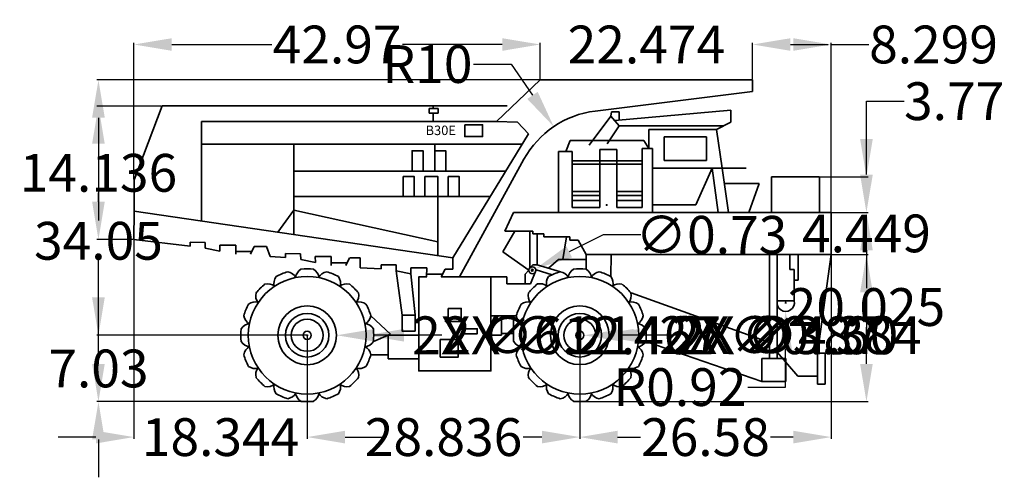
# Model space of a CAD drawing. Units: millimetres. Extents: x 52 to 156, y 12 to 60.
import ezdxf

# ---------------------------------------------------------------- set-up
doc = ezdxf.new("R2010")
doc.units = ezdxf.units.MM
doc.header["$MEASUREMENT"] = 0
for name, color, linetype, lineweight in [('M-DIMS', 2, 'Continuous', 18), ('M-OUTL', 7, 'Continuous', 35), ('M-TEXT', 3, 'Continuous', 25), ('M-WHEL', 8, 'Continuous', 35)]:
    doc.layers.add(name, color=color, linetype=linetype, lineweight=lineweight)
doc.styles.get("Standard").update_dxf_attribs({"font": 'arial.ttf'})
doc.dimstyles.get("Standard").update_dxf_attribs({"dimtxt": 4, "dimasz": 4, "dimexe": 0.18, "dimexo": 0.0625, "dimgap": 0.09, "dimtad": 0, "dimtih": 1, "dimtoh": 1, "dimdec": 0, "dimzin": 0, "dimdsep": 46, "dimtxsty": 'Standard', "dimcen": 0.09, "dimadec": 0, "dimazin": 0, "dimtfac": 1, "dimtdec": 0, "dimtofl": 0, "dimtmove": 0, "dimatfit": 3, "dimfxl": 1, "dimtolj": 1, "dimtzin": 0, "dimarcsym": 0})

# ---------------------------------------------------------------- blocks, each defined once
blk = doc.blocks.new('*U3')
for p, q in [((-6.73, -0.78), (-6.43, 0.09)), ((-4.89, 0.27), (-4.78, -0.69)), ((-3.11, -0.49), (-3.19, 0.15)), ((-3.19, 0.15), (-1.61, 0.02)), ((-1.61, 0.02), (-1.53, -0.6)), ((0.05, -0.42), (0, 0)), ((-4.86, -0.01), (-6.54, -0.21)), ((-4.78, -0.69), (-3.11, -0.49)), ((-1.53, -0.6), (0.05, -0.42))]:
    blk.add_line(p, q)
blk = doc.blocks.new('*U4')
at = {"layer": 'M-OUTL', "color": 0, "linetype": 'ByBlock', "lineweight": -2, "transparency": 16777216, "rotation": 173.2489355326982}
for p in [(70.14, 36.17), (80.23, 34.97), (90.33, 33.78)]:
    blk.add_blockref('*U3', p, dxfattribs=at)
blk = doc.blocks.new('*U1')
for centre, radius, start, end in [((0, -0.63), 1.25, 122.4091, 172.2725), ((0, -6.57), 7.03, 84.5202, 95.4798), ((0, -0.63), 1.25, 7.7275, 57.5909)]:
    blk.add_arc(centre, radius, start, end)
blk = doc.blocks.new('*U2')
at = {"color": 0, "linetype": 'ByBlock', "lineweight": -2, "transparency": 16777216}
for p, rotation in [((21.9, 20.49), 22.49999999999999), ((26.93, 20.49), 337.5), ((19.77, 19.07), 45.00000000000001), ((29.06, 19.07), 315), ((18.35, 16.94), 67.5), ((30.49, 16.94), 292.5), ((17.85, 14.43), 90), ((30.99, 14.43), 270), ((18.35, 11.91), 112.5), ((30.49, 11.91), 247.5), ((19.77, 9.78), 135), ((29.06, 9.78), 225), ((21.9, 8.36), 157.5), ((26.93, 8.36), 202.4999999999999), ((24.42, 7.86), 180)]:
    blk.add_blockref('*U1', p, dxfattribs=dict(at, rotation=rotation))
blk.add_blockref('*U1', (24.42, 21), dxfattribs=at)
blk = doc.blocks.new('WHEEL-TYRE')
for radius in [6.23, 3.11, 2.3, 1.69, 0.434]:
    blk.add_circle((6.23, 6.23), radius)
blk.add_blockref('*U2', (-18.18, -8.19))
blk = doc.blocks.new('*D6')
at = {"layer": 'Defpoints', "color": 0, "transparency": 16777216}
for p in [(107.16, 57.52), (107.16, 53.77), (64.19, 43.2)]:
    blk.add_point(p, dxfattribs=at)
at = {"layer": 'M-DIMS', "color": 0, "lineweight": -2, "transparency": 16777216}
for p, q in [((64.19, 43.26), (64.19, 57.7)), ((68.19, 57.52), (78.76, 57.52)), ((103.16, 57.52), (92.6, 57.52)), ((107.16, 53.84), (107.16, 57.7))]:
    blk.add_line(p, q, dxfattribs=at)
at = {"layer": 'M-DIMS', "color": 0, "transparency": 16777216}
for points in [[(68.19, 58.18), (68.19, 56.85), (64.19, 57.52)], [(103.16, 58.18), (103.16, 56.85), (107.16, 57.52)]]:
    blk.add_solid(points, dxfattribs=at)
at = {"layer": 'M-DIMS', "color": 0, "transparency": 16777216, "insert": (85.68, 57.52), "char_height": 4, "attachment_point": 5}
blk.add_mtext('\\A1;42.97', dxfattribs=at)
blk = doc.blocks.new('*D7')
at = {"layer": 'Defpoints', "color": 0, "transparency": 16777216}
for p in [(129.64, 57.52), (107.16, 53.77), (129.64, 53.77)]:
    blk.add_point(p, dxfattribs=at)
at = {"layer": 'M-DIMS', "color": 0, "lineweight": -2, "transparency": 16777216}
for p, q in [((103.16, 57.52), (99.16, 57.52)), ((107.16, 53.84), (107.16, 57.7)), ((129.64, 53.84), (129.64, 57.7)), ((133.64, 57.52), (137.64, 57.52))]:
    blk.add_line(p, q, dxfattribs=at)
at = {"layer": 'M-DIMS', "color": 0, "transparency": 16777216}
for points in [[(103.16, 58.18), (103.16, 56.85), (107.16, 57.52)], [(133.64, 58.18), (133.64, 56.85), (129.64, 57.52)]]:
    blk.add_solid(points, dxfattribs=at)
at = {"layer": 'M-DIMS', "color": 0, "transparency": 16777216, "insert": (118.4, 57.52), "char_height": 4, "attachment_point": 5}
blk.add_mtext('\\A1;22.474', dxfattribs=at)
blk = doc.blocks.new('*D8')
at = {"layer": 'Defpoints', "color": 0, "transparency": 16777216}
for p in [(137.94, 57.52), (129.64, 53.77), (137.94, 39.75)]:
    blk.add_point(p, dxfattribs=at)
at = {"layer": 'M-DIMS', "color": 0, "lineweight": -2, "transparency": 16777216}
for p, q in [((129.64, 53.84), (129.64, 57.7)), ((133.64, 57.52), (133.94, 57.52)), ((137.94, 39.81), (137.94, 57.7)), ((137.94, 57.52), (141.94, 57.52))]:
    blk.add_line(p, q, dxfattribs=at)
at = {"layer": 'M-DIMS', "color": 0, "transparency": 16777216}
for points in [[(133.64, 58.18), (133.64, 56.85), (129.64, 57.52)], [(133.94, 58.18), (133.94, 56.85), (137.94, 57.52)]]:
    blk.add_solid(points, dxfattribs=at)
at = {"layer": 'M-DIMS', "color": 0, "transparency": 16777216, "insert": (148.78, 57.52), "char_height": 4, "attachment_point": 5}
blk.add_mtext('\\A1;8.299', dxfattribs=at)
blk = doc.blocks.new('*D9')
at = {"layer": 'Defpoints', "color": 0, "transparency": 16777216}
for p in [(64.17, 36.88), (82.52, 26.75), (82.52, 15.98)]:
    blk.add_point(p, dxfattribs=at)
at = {"layer": 'M-DIMS', "color": 0, "lineweight": -2, "transparency": 16777216}
for p, q in [((64.17, 36.81), (64.17, 15.8)), ((82.52, 26.69), (82.52, 15.8)), ((60.17, 15.98), (56.17, 15.98)), ((86.52, 15.98), (90.52, 15.98))]:
    blk.add_line(p, q, dxfattribs=at)
at = {"layer": 'M-DIMS', "color": 0, "transparency": 16777216}
for points in [[(60.17, 16.65), (60.17, 15.31), (64.17, 15.98)], [(86.52, 16.65), (86.52, 15.31), (82.52, 15.98)]]:
    blk.add_solid(points, dxfattribs=at)
at = {"layer": 'M-DIMS', "color": 0, "transparency": 16777216, "insert": (73.35, 15.98), "char_height": 4, "attachment_point": 5}
blk.add_mtext('\\A1;18.344', dxfattribs=at)
blk = doc.blocks.new('*D10')
at = {"layer": 'Defpoints', "color": 0, "transparency": 16777216}
for p in [(82.52, 26.75), (111.35, 26.75), (111.35, 15.98)]:
    blk.add_point(p, dxfattribs=at)
at = {"layer": 'M-DIMS', "color": 0, "lineweight": -2, "transparency": 16777216}
for p, q in [((82.52, 26.69), (82.52, 15.8)), ((111.35, 26.69), (111.35, 15.8)), ((86.52, 15.98), (88.51, 15.98)), ((107.35, 15.98), (105.36, 15.98))]:
    blk.add_line(p, q, dxfattribs=at)
at = {"layer": 'M-DIMS', "color": 0, "transparency": 16777216}
for points in [[(86.52, 16.65), (86.52, 15.31), (82.52, 15.98)], [(107.35, 16.65), (107.35, 15.31), (111.35, 15.98)]]:
    blk.add_solid(points, dxfattribs=at)
at = {"layer": 'M-DIMS', "color": 0, "transparency": 16777216, "insert": (96.94, 15.98), "char_height": 4, "attachment_point": 5}
blk.add_mtext('\\A1;28.836', dxfattribs=at)
blk = doc.blocks.new('*D11')
at = {"layer": 'Defpoints', "color": 0, "transparency": 16777216}
for p in [(137.94, 35.3), (111.35, 26.75), (137.94, 15.98)]:
    blk.add_point(p, dxfattribs=at)
at = {"layer": 'M-DIMS', "color": 0, "lineweight": -2, "transparency": 16777216}
for p, q in [((137.94, 35.24), (137.94, 15.8)), ((111.35, 26.69), (111.35, 15.8)), ((115.35, 15.98), (117.77, 15.98)), ((133.94, 15.98), (131.52, 15.98))]:
    blk.add_line(p, q, dxfattribs=at)
at = {"layer": 'M-DIMS', "color": 0, "transparency": 16777216}
for points in [[(115.35, 16.65), (115.35, 15.31), (111.35, 15.98)], [(133.94, 16.65), (133.94, 15.31), (137.94, 15.98)]]:
    blk.add_solid(points, dxfattribs=at)
at = {"layer": 'M-DIMS', "color": 0, "transparency": 16777216, "insert": (124.65, 15.98), "char_height": 4, "attachment_point": 5}
blk.add_mtext('\\A1;26.58', dxfattribs=at)
blk = doc.blocks.new('*D12')
at = {"layer": 'Defpoints', "color": 0, "transparency": 16777216}
for p in [(60.43, 53.77), (107.16, 53.77), (82.52, 19.73)]:
    blk.add_point(p, dxfattribs=at)
at = {"layer": 'M-DIMS', "color": 0, "lineweight": -2, "transparency": 16777216}
for p, q in [((107.1, 53.77), (60.25, 53.77)), ((60.43, 49.77), (60.43, 38.88)), ((60.43, 23.73), (60.43, 34.62)), ((82.46, 19.73), (60.25, 19.73))]:
    blk.add_line(p, q, dxfattribs=at)
at = {"layer": 'M-DIMS', "color": 0, "transparency": 16777216}
for points in [[(59.76, 49.77), (61.1, 49.77), (60.43, 53.77)], [(59.76, 23.73), (61.1, 23.73), (60.43, 19.73)]]:
    blk.add_solid(points, dxfattribs=at)
at = {"layer": 'M-DIMS', "color": 0, "transparency": 16777216, "insert": (60.43, 36.75), "char_height": 4, "attachment_point": 5}
blk.add_mtext('\\A1;34.05', dxfattribs=at)
blk = doc.blocks.new('*D13')
at = {"layer": 'Defpoints', "color": 0, "transparency": 16777216}
for p in [(60.43, 26.75), (82.52, 26.75), (82.52, 19.73)]:
    blk.add_point(p, dxfattribs=at)
at = {"layer": 'M-DIMS', "color": 0, "lineweight": -2, "transparency": 16777216}
for p, q in [((60.43, 30.75), (60.43, 34.75)), ((82.46, 26.75), (60.25, 26.75)), ((82.46, 19.73), (60.25, 19.73)), ((60.43, 15.73), (60.43, 11.73))]:
    blk.add_line(p, q, dxfattribs=at)
at = {"layer": 'M-DIMS', "color": 0, "transparency": 16777216}
for points in [[(59.76, 30.75), (61.1, 30.75), (60.43, 26.75)], [(59.76, 15.73), (61.1, 15.73), (60.43, 19.73)]]:
    blk.add_solid(points, dxfattribs=at)
at = {"layer": 'M-DIMS', "color": 0, "transparency": 16777216, "insert": (60.43, 23.24), "char_height": 4, "attachment_point": 5}
blk.add_mtext('\\A1;7.03', dxfattribs=at)
blk = doc.blocks.new('*D14')
at = {"layer": 'Defpoints', "color": 0, "transparency": 16777216}
for p in [(60.43, 51.01), (67.17, 51.01), (64.17, 36.88)]:
    blk.add_point(p, dxfattribs=at)
at = {"layer": 'M-DIMS', "color": 0, "lineweight": -2, "transparency": 16777216}
for p, q in [((67.11, 51.01), (60.25, 51.01)), ((60.43, 47.01), (60.43, 46.08)), ((60.43, 40.88), (60.43, 41.81)), ((64.11, 36.88), (60.25, 36.88))]:
    blk.add_line(p, q, dxfattribs=at)
at = {"layer": 'M-DIMS', "color": 0, "transparency": 16777216}
for points in [[(59.76, 47.01), (61.1, 47.01), (60.43, 51.01)], [(59.76, 40.88), (61.1, 40.88), (60.43, 36.88)]]:
    blk.add_solid(points, dxfattribs=at)
at = {"layer": 'M-DIMS', "color": 0, "transparency": 16777216, "insert": (60.43, 43.94), "char_height": 4, "attachment_point": 5}
blk.add_mtext('\\A1;14.136', dxfattribs=at)
blk = doc.blocks.new('*D15')
at = {"layer": 'Defpoints', "color": 0, "transparency": 16777216}
for p in [(137.94, 39.75), (141.68, 39.75), (137.94, 35.3)]:
    blk.add_point(p, dxfattribs=at)
at = {"layer": 'M-DIMS', "color": 0, "lineweight": -2, "transparency": 16777216}
for p, q in [((141.68, 43.75), (141.68, 47.75)), ((138, 39.75), (141.86, 39.75)), ((138, 35.3), (141.86, 35.3)), ((141.68, 31.3), (141.68, 27.3))]:
    blk.add_line(p, q, dxfattribs=at)
at = {"layer": 'M-DIMS', "color": 0, "transparency": 16777216}
for points in [[(141.01, 43.75), (142.35, 43.75), (141.68, 39.75)], [(141.01, 31.3), (142.35, 31.3), (141.68, 35.3)]]:
    blk.add_solid(points, dxfattribs=at)
at = {"layer": 'M-DIMS', "color": 0, "transparency": 16777216, "insert": (141.68, 37.53), "char_height": 4, "attachment_point": 5}
blk.add_mtext('\\A1;4.449', dxfattribs=at)
blk = doc.blocks.new('*D16')
at = {"layer": 'Defpoints', "color": 0, "transparency": 16777216}
for p in [(137.94, 39.75), (141.68, 39.75), (111.35, 19.73)]:
    blk.add_point(p, dxfattribs=at)
at = {"layer": 'M-DIMS', "color": 0, "lineweight": -2, "transparency": 16777216}
for p, q in [((138, 39.75), (141.86, 39.75)), ((141.68, 35.75), (141.68, 31.87)), ((141.68, 23.73), (141.68, 27.61)), ((111.42, 19.73), (141.86, 19.73))]:
    blk.add_line(p, q, dxfattribs=at)
at = {"layer": 'M-DIMS', "color": 0, "transparency": 16777216}
for points in [[(141.01, 35.75), (142.35, 35.75), (141.68, 39.75)], [(141.01, 23.73), (142.35, 23.73), (141.68, 19.73)]]:
    blk.add_solid(points, dxfattribs=at)
at = {"layer": 'M-DIMS', "color": 0, "transparency": 16777216, "insert": (141.68, 29.74), "char_height": 4, "attachment_point": 5}
blk.add_mtext('\\A1;20.025', dxfattribs=at)
blk = doc.blocks.new('*D17')
at = {"layer": 'Defpoints', "color": 0, "transparency": 16777216}
for p in [(136.7, 43.52), (141.68, 43.52), (137.94, 39.75)]:
    blk.add_point(p, dxfattribs=at)
at = {"layer": 'M-DIMS', "color": 0, "lineweight": -2, "transparency": 16777216}
for p, q in [((141.68, 47.52), (141.68, 51.52)), ((141.68, 51.52), (145.68, 51.52)), ((136.77, 43.52), (141.86, 43.52)), ((138, 39.75), (141.86, 39.75)), ((141.68, 35.75), (141.68, 31.75))]:
    blk.add_line(p, q, dxfattribs=at)
at = {"layer": 'M-DIMS', "color": 0, "transparency": 16777216}
for points in [[(141.01, 47.52), (142.35, 47.52), (141.68, 43.52)], [(141.01, 35.75), (142.35, 35.75), (141.68, 39.75)]]:
    blk.add_solid(points, dxfattribs=at)
at = {"layer": 'M-DIMS', "color": 0, "transparency": 16777216, "insert": (150.96, 51.52), "char_height": 4, "attachment_point": 5}
blk.add_mtext('\\A1;3.77', dxfattribs=at)
blk = doc.blocks.new('*D18')
at = {"layer": 'Defpoints', "color": 0, "transparency": 16777216}
for p in [(76.28, 26.75), (88.75, 26.75)]:
    blk.add_point(p, dxfattribs=at)
at = {"layer": 'M-DIMS', "color": 0, "lineweight": -2, "transparency": 16777216}
for p, q in [((82.43, 26.75), (82.61, 26.75)), ((82.52, 26.66), (82.52, 26.84)), ((96.75, 26.75), (92.75, 26.75))]:
    blk.add_line(p, q, dxfattribs=at)
at = {"layer": 'M-DIMS', "color": 0, "transparency": 16777216}
blk.add_solid([(92.75, 27.42), (92.75, 26.09), (88.75, 26.75)], dxfattribs=at)
at = {"layer": 'M-DIMS', "color": 0, "transparency": 16777216, "insert": (111.55, 26.75), "char_height": 4, "attachment_point": 5}
blk.add_mtext('\\A1;2X ∅12.467', dxfattribs=at)
blk = doc.blocks.new('*D19')
at = {"layer": 'Defpoints', "color": 0, "transparency": 16777216}
for p in [(79.41, 26.75), (85.63, 26.75)]:
    blk.add_point(p, dxfattribs=at)
at = {"layer": 'M-DIMS', "color": 0, "lineweight": -2, "transparency": 16777216}
for p, q in [((82.43, 26.75), (82.61, 26.75)), ((82.52, 26.66), (82.52, 26.84)), ((93.63, 26.75), (89.63, 26.75))]:
    blk.add_line(p, q, dxfattribs=at)
at = {"layer": 'M-DIMS', "color": 0, "transparency": 16777216}
blk.add_solid([(89.63, 27.42), (89.63, 26.09), (85.63, 26.75)], dxfattribs=at)
at = {"layer": 'M-DIMS', "color": 0, "transparency": 16777216, "insert": (106.86, 26.75), "char_height": 4, "attachment_point": 5}
blk.add_mtext('\\A1;2X ∅6.214', dxfattribs=at)
blk = doc.blocks.new('*D20')
at = {"layer": 'Defpoints', "color": 0, "transparency": 16777216}
for p in [(109.05, 26.75), (113.65, 26.75)]:
    blk.add_point(p, dxfattribs=at)
at = {"layer": 'M-DIMS', "color": 0, "lineweight": -2, "transparency": 16777216}
for p, q in [((111.26, 26.75), (111.44, 26.75)), ((111.35, 26.66), (111.35, 26.84)), ((121.65, 26.75), (117.65, 26.75))]:
    blk.add_line(p, q, dxfattribs=at)
at = {"layer": 'M-DIMS', "color": 0, "transparency": 16777216}
blk.add_solid([(117.65, 27.42), (117.65, 26.09), (113.65, 26.75)], dxfattribs=at)
at = {"layer": 'M-DIMS', "color": 0, "transparency": 16777216, "insert": (133.33, 26.75), "char_height": 4, "attachment_point": 5}
blk.add_mtext('\\A1;2X ∅4.60', dxfattribs=at)
blk = doc.blocks.new('*D21')
at = {"layer": 'Defpoints', "color": 0, "transparency": 16777216}
for p in [(109.66, 26.75), (113.05, 26.75)]:
    blk.add_point(p, dxfattribs=at)
at = {"layer": 'M-DIMS', "color": 0, "lineweight": -2, "transparency": 16777216}
for p, q in [((111.26, 26.75), (111.44, 26.75)), ((111.35, 26.66), (111.35, 26.84)), ((121.05, 26.76), (117.05, 26.76))]:
    blk.add_line(p, q, dxfattribs=at)
at = {"layer": 'M-DIMS', "color": 0, "transparency": 16777216}
blk.add_solid([(117.05, 27.42), (117.05, 26.09), (113.05, 26.75)], dxfattribs=at)
at = {"layer": 'M-DIMS', "color": 0, "transparency": 16777216, "insert": (134.28, 26.76), "char_height": 4, "attachment_point": 5}
blk.add_mtext('\\A1;2X ∅3.384', dxfattribs=at)
blk = doc.blocks.new('*D22')
at = {"layer": 'Defpoints', "color": 0, "transparency": 16777216}
for p in [(110.92, 26.75), (111.79, 26.75)]:
    blk.add_point(p, dxfattribs=at)
at = {"layer": 'M-DIMS', "color": 0, "lineweight": -2, "transparency": 16777216}
for p, q in [((111.26, 26.75), (111.44, 26.75)), ((111.35, 26.66), (111.35, 26.84)), ((119.79, 26.76), (115.79, 26.76))]:
    blk.add_line(p, q, dxfattribs=at)
at = {"layer": 'M-DIMS', "color": 0, "transparency": 16777216}
blk.add_solid([(115.79, 27.42), (115.79, 26.09), (111.79, 26.75)], dxfattribs=at)
at = {"layer": 'M-DIMS', "color": 0, "transparency": 16777216, "insert": (131.47, 26.76), "char_height": 4, "attachment_point": 5}
blk.add_mtext('\\A1;2X ∅0.87', dxfattribs=at)
blk = doc.blocks.new('*D23')
at = {"layer": 'Defpoints', "color": 0, "transparency": 16777216}
for p in [(108.6, 48.83), (114.21, 40.55)]:
    blk.add_point(p, dxfattribs=at)
at = {"layer": 'M-DIMS', "color": 0, "lineweight": -2, "transparency": 16777216}
for p, q in [((100.1, 55.45), (104.1, 55.45)), ((104.1, 55.45), (106.35, 52.14)), ((114.21, 40.46), (114.21, 40.64)), ((114.12, 40.55), (114.3, 40.55))]:
    blk.add_line(p, q, dxfattribs=at)
at = {"layer": 'M-DIMS', "color": 0, "transparency": 16777216}
blk.add_solid([(106.9, 52.51), (105.8, 51.76), (108.6, 48.83)], dxfattribs=at)
at = {"layer": 'M-DIMS', "color": 0, "transparency": 16777216, "insert": (95.24, 55.45), "char_height": 4, "attachment_point": 5}
blk.add_mtext('\\A1;R10', dxfattribs=at)
blk = doc.blocks.new('*D24')
at = {"layer": 'Defpoints', "color": 0, "transparency": 16777216}
for p in [(133.14, 30.19), (133.14, 29.27)]:
    blk.add_point(p, dxfattribs=at)
at = {"layer": 'M-DIMS', "color": 0, "lineweight": -2, "transparency": 16777216}
for p, q in [((133.14, 30.1), (133.14, 30.28)), ((133.05, 30.19), (133.23, 30.19)), ((133.13, 21.27), (133.13, 25.27)), ((129.13, 21.27), (133.13, 21.27))]:
    blk.add_line(p, q, dxfattribs=at)
at = {"layer": 'M-DIMS', "color": 0, "transparency": 16777216}
blk.add_solid([(132.47, 25.27), (133.8, 25.27), (133.14, 29.27)], dxfattribs=at)
at = {"layer": 'M-DIMS', "color": 0, "transparency": 16777216, "insert": (121.95, 21.27), "char_height": 4, "attachment_point": 5}
blk.add_mtext('\\A1;R0.92', dxfattribs=at)
blk = doc.blocks.new('*D25')
at = {"layer": 'Defpoints', "color": 0, "transparency": 16777216}
for p in [(106.01, 33.46), (106.67, 33.79)]:
    blk.add_point(p, dxfattribs=at)
at = {"layer": 'M-DIMS', "color": 0, "lineweight": -2, "transparency": 16777216}
for p, q in [((113.82, 37.38), (110.24, 35.59)), ((117.82, 37.38), (113.82, 37.38)), ((106.25, 33.63), (106.43, 33.63)), ((106.34, 33.54), (106.34, 33.72))]:
    blk.add_line(p, q, dxfattribs=at)
at = {"layer": 'M-DIMS', "color": 0, "transparency": 16777216}
blk.add_solid([(109.94, 36.18), (110.54, 34.99), (106.67, 33.79)], dxfattribs=at)
at = {"layer": 'M-DIMS', "color": 0, "transparency": 16777216, "insert": (125.28, 37.38), "char_height": 4, "attachment_point": 5}
blk.add_mtext('\\A1;∅0.73', dxfattribs=at)

msp = doc.modelspace()

# ---------------------------------------------------------------- linework, layer by layer
at = {"layer": 'M-OUTL'}
for p, q in [((107.1632, 53.7726), (102.5408, 49.3664)), ((129.6372, 53.7726), (107.1632, 53.7726)), ((129.6372, 52.5516), (129.6372, 53.7726)), ((112.9751, 50.4757), (129.6372, 52.5516)), ((67.1683, 51.0117), (64.1936, 43.1988)), ((103.6667, 51.0117), (67.1683, 51.0117)), ((95.8429, 50.7411), (95.4092, 50.7411)), ((95.4092, 50.7411), (96.3806, 50.7411)), ((95.4092, 50.2558), (95.4092, 50.7411)), ((96.3806, 50.2558), (95.4092, 50.2558)), ((95.8429, 51.0117), (95.8429, 50.7411)), ((95.8576, 49.3664), (95.8576, 50.2558)), ((96.3806, 50.7411), (96.3806, 50.2558)), ((114.6367, 49.95), (114.7108, 50.3838)), ((114.7108, 50.3838), (115.5029, 50.3838)), ((127.3175, 50.559), (115.0652, 49.459)), ((115.5029, 50.3838), (115.5029, 49.4983)), ((127.3175, 49.3094), (127.3175, 50.559)), ((102.5408, 49.3664), (71.3461, 49.3664)), ((71.3461, 49.3664), (71.3461, 39.71)), ((104.7482, 49.2924), (102.5408, 49.3664)), ((105.9125, 48.0737), (104.7482, 49.2924)), ((112.3313, 46.8522), (114.6367, 49.95)), ((114.6367, 49.95), (115.5377, 48.9174)), ((125.8196, 48.5333), (127.3175, 49.3094)), ((97.9352, 34.9614), (105.9125, 48.0737)), ((115.5377, 48.9174), (114.2657, 47.0111)), ((114.2657, 47.0111), (115.5377, 48.9174)), ((115.5377, 48.9174), (126.561, 48.9174)), ((118.6701, 46.502), (118.6701, 48.5333)), ((118.6701, 48.5333), (125.8196, 48.5333)), ((126.561, 48.9174), (125.8196, 48.5333)), ((125.8196, 48.5333), (126.4109, 44.4448)), ((71.3461, 46.9695), (105.2407, 46.9695)), ((81.0868, 46.9695), (81.0868, 37.4209)), ((96.0115, 46.2741), (96.0115, 46.9695)), ((109.8691, 46.2129), (110.3523, 47.3619)), ((110.3523, 47.3619), (118.1208, 47.3619)), ((118.1208, 47.3619), (118.6701, 46.502)), ((120.285, 45.8155), (120.285, 47.7534)), ((120.285, 47.7534), (124.7553, 47.7534)), ((124.7553, 47.7534), (124.7553, 45.2483)), ((109.0949, 39.7505), (109.0949, 46.2129)), ((109.0949, 46.2129), (110.5336, 46.2129)), ((110.5336, 46.2129), (110.5336, 40.2574)), ((113.4796, 40.2574), (113.4796, 46.4183)), ((113.4796, 46.4183), (115.2608, 46.4183)), ((115.2608, 46.4183), (115.2608, 40.2666)), ((117.9511, 40.2666), (117.9511, 46.502)), ((117.9511, 46.502), (119.0592, 46.502)), ((119.0592, 46.502), (119.0592, 39.7505)), ((120.285, 45.8155), (120.285, 46.7608)), ((98.6158, 32.9353), (105.4474, 45.3681)), ((110.5336, 45.2044), (117.9511, 45.2044)), ((110.5336, 44.8484), (117.9511, 44.8484)), ((120.285, 45.2483), (120.285, 45.8155)), ((124.7553, 45.2483), (120.285, 45.2483)), ((81.0868, 44.1095), (103.5008, 44.1095)), ((126.4109, 44.4448), (119.0592, 44.4448)), ((123.62, 40.569), (125.3531, 44.4448)), ((125.3531, 44.4448), (125.9803, 39.7505)), ((126.4109, 44.4448), (128.9417, 44.4448)), ((126.4109, 44.4448), (127.0898, 39.7505)), ((64.1936, 43.1988), (64.1936, 39.8869)), ((126.6498, 42.7934), (130.3282, 42.7934)), ((130.3282, 42.7934), (129.2391, 39.7505)), ((131.6514, 39.7505), (131.6514, 43.5229)), ((131.6514, 43.5229), (136.7042, 43.5229)), ((136.7042, 43.5229), (136.7042, 39.7505)), ((110.5336, 41.9561), (113.4796, 41.9561)), ((115.2608, 41.9561), (117.9511, 41.9561)), ((96.3406, 41.424), (81.0868, 41.424)), ((81.0868, 41.424), (101.867, 41.424)), ((96.3406, 35.1942), (96.3406, 41.424)), ((110.5336, 41.5334), (113.4796, 41.5334)), ((110.5336, 40.9995), (113.4796, 40.9995)), ((115.2608, 41.5334), (117.9511, 41.5334)), ((115.2608, 40.9995), (117.9511, 40.9995)), ((64.1742, 36.8756), (64.1936, 39.8869)), ((64.1936, 39.8869), (97.9352, 34.9614)), ((71.3461, 39.71), (71.3461, 38.8428)), ((79.4256, 37.6634), (81.0868, 39.9871)), ((81.0868, 39.9871), (96.3406, 36.6458)), ((104.3372, 39.7505), (103.4196, 37.7757)), ((137.9361, 39.7505), (104.3372, 39.7505)), ((110.5336, 40.2574), (113.4796, 40.2574)), ((115.2608, 40.2666), (117.9511, 40.2666)), ((119.0592, 40.569), (123.62, 40.569)), ((137.9361, 35.3016), (137.9361, 39.7505)), ((103.2079, 35.5937), (104.4983, 37.7757)), ((103.4196, 37.7757), (106.3842, 37.7757)), ((106.0719, 33.8781), (106.0719, 37.7757)), ((106.3842, 37.7757), (106.3842, 37.4782)), ((70.1371, 36.1698), (64.1742, 36.8756)), ((96.3406, 36.6458), (96.3406, 35.1942)), ((106.3842, 37.4782), (107.5347, 37.4782)), ((106.8626, 34.2023), (106.8626, 37.4782)), ((107.5347, 37.4782), (107.5347, 37.1647)), ((107.5347, 37.1647), (110.2883, 37.1647)), ((109.5526, 34.7549), (109.9502, 37.1647)), ((110.2883, 37.1647), (110.2883, 36.7991)), ((110.2883, 36.7991), (111.1945, 36.7991)), ((111.1945, 36.7991), (112.0253, 35.3016)), ((76.9151, 36.1488), (77.3059, 36.1488)), ((77.1066, 36.1488), (78.222, 36.1488)), ((78.222, 36.1488), (78.6111, 35.1018)), ((105.9734, 33.6352), (103.2079, 35.5937)), ((78.6111, 35.1018), (80.2335, 34.9746)), ((87.0115, 34.9536), (88.1049, 34.9536)), ((88.1049, 34.9536), (88.1049, 33.9057)), ((97.9352, 34.9614), (97.9352, 33.7584)), ((109.103, 34.7549), (108.0498, 33.8484)), ((112.0253, 34.7549), (109.103, 34.7549)), ((112.0253, 33.7527), (112.0253, 35.3016)), ((112.0253, 35.3016), (114.6858, 35.3016)), ((114.6858, 35.3016), (114.6521, 32.9631)), ((114.6858, 35.3016), (137.9361, 35.3016)), ((131.4221, 24.2911), (131.4221, 35.3016)), ((132.2418, 35.3016), (132.2418, 30.3992)), ((133.5746, 33.7148), (133.5746, 35.3016)), ((134.4664, 32.5751), (134.4664, 35.3016)), ((136.5206, 24.8487), (137.9361, 35.3016)), ((88.1049, 33.9057), (90.33, 33.7794)), ((91.9248, 33.5697), (92.5527, 28.881)), ((97.9352, 33.7584), (97.108, 33.7584)), ((105.9734, 33.6352), (105.5715, 33.2206)), ((106.3747, 34.2023), (106.0719, 33.8781)), ((106.1529, 32.2078), (106.7517, 33.6704)), ((106.8626, 34.2023), (106.3747, 34.2023)), ((106.7517, 33.6704), (108.4232, 33.1448)), ((109.2963, 33.4769), (106.8626, 34.2023)), ((134.0308, 33.7148), (133.5746, 33.7148)), ((134.0308, 32.5751), (134.0308, 33.7148)), ((93.4777, 33.2552), (93.9309, 28.9047)), ((101.9464, 32.9353), (103.6355, 32.9353)), ((103.6355, 32.9353), (103.6355, 32.2078)), ((105.5715, 33.2206), (105.5715, 32.2078)), ((134.0308, 30.3992), (134.0308, 32.5751)), ((134.0308, 32.5751), (134.4664, 32.5751)), ((103.6355, 32.2078), (106.1529, 32.2078)), ((116.7768, 31.2284), (131.4221, 25.9797)), ((132.2418, 30.3992), (134.0308, 30.3992)), ((132.2418, 29.9834), (132.2418, 24.2911)), ((91.3304, 26.8567), (89.2402, 28.8127)), ((93.9309, 28.881), (93.9309, 28.9047)), ((104.632, 28.8127), (101.9464, 28.8127)), ((103.0749, 28.8127), (103.0749, 26.7549)), ((104.3262, 28.8127), (104.3262, 26.927)), ((89.5159, 26.0836), (91.3304, 26.8567)), ((94.3246, 26.7549), (91.0911, 26.7549)), ((91.0911, 26.7549), (91.0911, 24.2606)), ((101.9464, 26.7549), (103.0749, 26.7549)), ((104.3262, 26.927), (103.0749, 26.927)), ((130.6252, 21.8735), (118.3517, 26.0836)), ((89.2402, 24.6972), (91.0911, 24.6972)), ((91.0911, 24.2606), (94.3246, 24.2606)), ((130.6252, 24.2911), (133.1417, 24.2911)), ((130.6252, 21.8735), (130.6252, 24.2911)), ((132.2418, 24.9822), (134.4272, 22.4302)), ((133.1417, 24.2911), (133.1417, 21.8735)), ((137.3056, 24.8487), (136.5206, 24.8487)), ((136.5206, 24.8487), (136.5206, 22.4302)), ((137.3056, 21.5805), (137.3056, 24.8487)), ((134.4272, 22.4302), (136.5206, 22.4302)), ((136.5206, 22.4302), (136.5206, 21.5805)), ((133.1417, 21.8735), (130.6252, 21.8735)), ((136.5206, 21.5805), (137.3056, 21.5805))]:
    msp.add_line(p, q, dxfattribs=at)
for points in [[(99.1817, 49.0215), (101.0761, 49.0215), (101.0761, 47.7821), (99.1817, 47.7821)], [(96.3406, 41.424), (94.9754, 41.424), (94.9754, 43.5454), (96.3406, 43.5454)], [(97.4169, 29.6023), (98.809, 29.6023), (98.809, 28.2112), (97.4169, 28.2112)], [(92.5527, 28.881), (93.9309, 28.881), (93.9309, 27.1953), (92.5527, 27.1953)], [(98.9511, 27.4448), (100.5137, 27.4448), (100.5137, 26.9054), (98.9511, 26.9054)], [(96.5955, 26.292), (98.4976, 26.292), (98.4976, 24.4367), (96.5955, 24.4367)]]:
    msp.add_lwpolyline(points, close=True, dxfattribs=at)
for points in [[(93.6115, 44.1527), (93.6115, 46.2741), (94.774, 46.2741), (94.774, 44.1527)], [(96.0115, 44.1527), (96.0115, 46.2741), (97.174, 46.2741), (97.174, 44.1527)], [(92.6749, 41.424), (92.6749, 43.5454), (93.8374, 43.5454), (93.8374, 41.424)], [(97.4456, 41.424), (97.4456, 43.5454), (98.6081, 43.5454), (98.6081, 41.424)], [(96.7061, 32.9353), (101.9464, 32.9353), (101.9464, 22.9777), (94.3246, 22.9777), (94.3246, 32.9353), (95.1564, 32.9353)]]:
    msp.add_lwpolyline(points, dxfattribs=at)
for centre, radius in [((106.3392, 33.6284), 0.3658), ((106.3275, 33.6347), 0.0974)]:
    msp.add_circle(centre, radius, dxfattribs=at)
for centre, radius, start, end in [((114.2115, 40.5524), 10, 97.102014, 151.212079), ((133.1363, 30.1913), 0.9184, 166.916665, 13.083335)]:
    msp.add_arc(centre, radius, start, end, dxfattribs=at)

# ---------------------------------------------------------------- block references
msp.add_blockref('*U4', (0, 0), dxfattribs=at)
at = {"layer": 'M-WHEL', "rotation": 112.5}
msp.add_blockref('WHEEL-TYRE', (119.4985, 23.3814), dxfattribs=at)
at = {"layer": 'M-WHEL'}
msp.add_blockref('WHEEL-TYRE', (76.2847, 20.5214), dxfattribs=at)

# ---------------------------------------------------------------- texts
at = {"layer": 'M-TEXT', "insert": (95.0374, 48.9354), "char_height": 1, "attachment_point": 1}
msp.add_mtext_dynamic_manual_height_columns('B30E', width=0.380493, gutter_width=1, heights=[0], dxfattribs=at)

# ---------------------------------------------------------------- dimensions: what is measured, and where the dimension line sits
at = {"layer": 'M-DIMS'}
for base, p1, p2, override, picture, middle in [((107.1632, 57.5176), (64.1936, 43.1988), (107.1632, 53.7726), {"dimdec": 2, "dimlfac": 1, "dimrnd": 0, "dimzin": 0, "dimdsep": 46, "dimlunit": 2}, '*D6', (85.6784, 57.5176)), ((129.6372, 57.5176), (107.1632, 53.7726), (129.6372, 53.7726), {"dimdec": 3, "dimlfac": 1, "dimrnd": 0, "dimzin": 0, "dimdsep": 46, "dimlunit": 2}, '*D7', (118.4002, 57.5176)), ((137.9361, 57.5176), (129.6372, 53.7726), (137.9361, 39.7505), {"dimdec": 3, "dimlfac": 1, "dimrnd": 0, "dimzin": 0, "dimdsep": 46, "dimlunit": 2}, '*D8', (148.7819, 57.5176)), ((82.5182, 15.9801), (64.1742, 36.8756), (82.5182, 26.7549), {"dimdec": 3, "dimlfac": 1, "dimrnd": 0, "dimzin": 0, "dimdsep": 46, "dimlunit": 2}, '*D9', (73.3462, 15.9801)), ((137.9361, 15.9801), (111.354, 26.7549), (137.9361, 35.3016), {"dimdec": 2, "dimlfac": 1, "dimrnd": 0, "dimzin": 0, "dimdsep": 46, "dimlunit": 2}, '*D11', (124.6451, 15.9801)), ((111.354, 15.9801), (82.5182, 26.7549), (111.354, 26.7549), {"dimdec": 3, "dimlfac": 1, "dimrnd": 0, "dimzin": 0, "dimdsep": 46, "dimlunit": 2}, '*D10', (96.9361, 15.9801))]:
    dim = msp.add_linear_dim(base=base, p1=p1, p2=p2, dimstyle='Standard', override=override, dxfattribs=at)
    dim.commit()
    dim.dimension.update_dxf_attribs({"geometry": picture, "text_midpoint": middle})
for center, mpoint, override, picture, middle in [((114.2115, 40.5524), (108.5968, 48.8273), {"dimdec": 0, "dimlfac": 1, "dimrnd": 0, "dimzin": 0, "dimdsep": 46, "dimlunit": 2}, '*D23', (95.2428, 55.4473)), ((133.1363, 30.1913), (133.136, 29.2729), {"dimdec": 2, "dimlfac": 1, "dimrnd": 0, "dimzin": 0, "dimdsep": 46, "dimlunit": 2}, '*D24', (121.9548, 21.2729))]:
    dim = msp.add_radius_dim(center=center, mpoint=mpoint, dimstyle='Standard', override=override, dxfattribs=at)
    dim.commit()
    dim.dimension.update_dxf_attribs({"geometry": picture, "text_midpoint": middle})
for base, p1, p2, override, picture, middle in [((60.4292, 53.7726), (82.5182, 19.7251), (107.1632, 53.7726), {"dimdec": 2, "dimlfac": 1, "dimrnd": 0, "dimzin": 0, "dimdsep": 46, "dimlunit": 2}, '*D12', (60.4292, 36.7489)), ((141.6811, 43.5229), (137.9361, 39.7505), (136.7042, 43.5229), {"dimdec": 2, "dimlfac": 1, "dimrnd": 0, "dimzin": 0, "dimdsep": 46, "dimlunit": 2}, '*D17', (150.9649, 51.5229)), ((60.4292, 51.0117), (64.1742, 36.8756), (67.1683, 51.0117), {"dimdec": 3, "dimlfac": 1, "dimrnd": 0, "dimzin": 0, "dimdsep": 46, "dimlunit": 2}, '*D14', (60.4292, 43.9436)), ((141.6811, 39.7505), (137.9361, 35.3016), (137.9361, 39.7505), {"dimdec": 3, "dimlfac": 1, "dimrnd": 0, "dimzin": 0, "dimdsep": 46, "dimlunit": 2}, '*D15', (141.6811, 37.5261)), ((141.6811, 39.7505), (111.354, 19.7251), (137.9361, 39.7505), {"dimdec": 3, "dimlfac": 1, "dimrnd": 0, "dimzin": 0, "dimdsep": 46, "dimlunit": 2}, '*D16', (141.6811, 29.7378)), ((60.4292, 26.7549), (82.5182, 19.7251), (82.5182, 26.7549), {"dimdec": 2, "dimlfac": 1, "dimrnd": 0, "dimzin": 0, "dimdsep": 46, "dimlunit": 2}, '*D13', (60.4292, 23.24))]:
    dim = msp.add_linear_dim(base=base, p1=p1, p2=p2, angle=90, dimstyle='Standard', override=override, dxfattribs=at)
    dim.commit()
    dim.dimension.update_dxf_attribs({"geometry": picture, "text_midpoint": middle})
dim = msp.add_diameter_dim_2p(p1=(106.0122, 33.4643), p2=(106.6662, 33.7925), dimstyle='Standard', override={"dimdec": 2, "dimlfac": 1, "dimrnd": 0, "dimzin": 0, "dimdsep": 46, "dimlunit": 2}, dxfattribs=at)
dim.commit()
dim.dimension.update_dxf_attribs({"geometry": '*D25', "text_midpoint": (125.2773, 37.381), "dimtype": 163})
for p1, p2, picture, middle in [((76.2847, 26.7549), (88.7517, 26.755), '*D18', (96.7517, 26.7551)), ((109.6619, 26.7549), (113.0461, 26.755), '*D21', (121.0461, 26.7552))]:
    dim = msp.add_diameter_dim_2p(p1=p1, p2=p2, text='2X <>', dimstyle='Standard', override={"dimdec": 3, "dimlfac": 1, "dimrnd": 0, "dimzin": 0, "dimdsep": 46, "dimlunit": 2}, dxfattribs=at)
    dim.commit()
    dim.dimension.update_dxf_attribs({"geometry": picture, "text_midpoint": middle})
for p1, p2, override, picture, middle in [((79.4111, 26.7549), (85.6253, 26.755), {"dimdec": 3, "dimlfac": 1, "dimrnd": 0, "dimzin": 0, "dimdsep": 46, "dimlunit": 2}, '*D19', (93.6253, 26.7551)), ((109.0547, 26.7549), (113.6532, 26.755), {"dimdec": 2, "dimlfac": 1, "dimrnd": 0, "dimzin": 0, "dimdsep": 46, "dimlunit": 2}, '*D20', (121.6532, 26.7552)), ((110.9198, 26.7549), (111.7881, 26.755), {"dimdec": 2, "dimlfac": 1, "dimrnd": 0, "dimzin": 0, "dimdsep": 46, "dimlunit": 2}, '*D22', (119.7881, 26.7559))]:
    dim = msp.add_diameter_dim_2p(p1=p1, p2=p2, text='2X <>', dimstyle='Standard', override=override, dxfattribs=at)
    dim.commit()
    dim.dimension.update_dxf_attribs({"geometry": picture, "text_midpoint": middle, "dimtype": 163})

doc.saveas('drawing.dxf')
